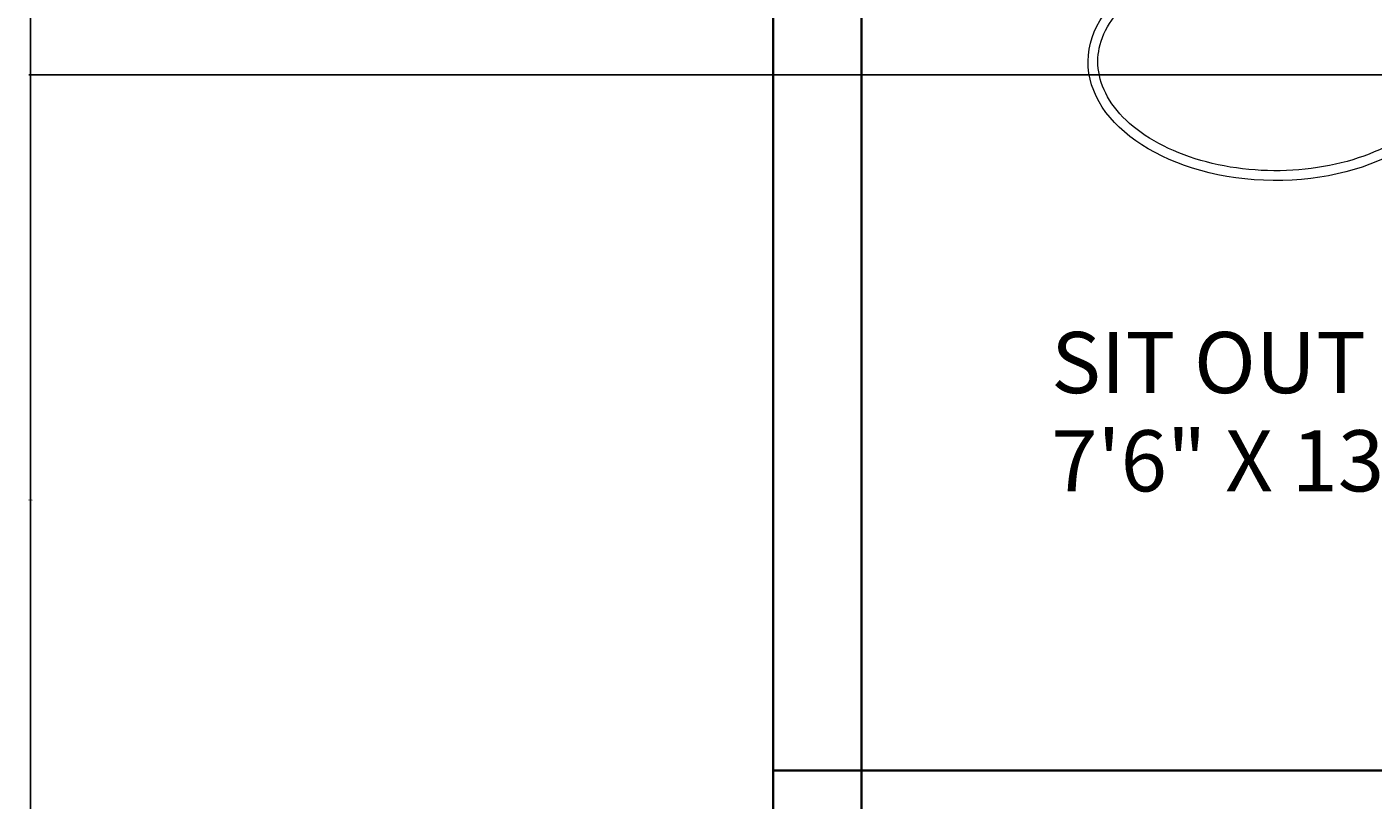
# Model space of a CAD drawing. Units: inches. Extents: x -61 to 1599, y -1316 to 257.
# Tile 14 of 204: x -61 to 76, y -947 to -868. Entities that reach past the tile are written whole.
import ezdxf

# ---------------------------------------------------------------- set-up
doc = ezdxf.new("R2010")
doc.units = ezdxf.units.IN
doc.header["$MEASUREMENT"] = 0
for name, color, linetype, lineweight in [('A-ANNO-DIMS', 2, 'Continuous', 18), ('A-AREA-IDEN', 1, 'Continuous', 18), ('FURNITURE', 83, 'Continuous', 18), ('WALLS', 4, 'Continuous', 35)]:
    doc.layers.add(name, color=color, linetype=linetype, lineweight=lineweight)
doc.styles.get("Standard").update_dxf_attribs({"font": 'arial.ttf'})
doc.dimstyles.get("Standard").update_dxf_attribs({"dimtxt": 0.18, "dimasz": 0.18, "dimexe": 0.18, "dimexo": 0.0625, "dimgap": 0.09, "dimtad": 0, "dimtih": 1, "dimtoh": 1, "dimdec": 0, "dimzin": 0, "dimdsep": 46, "dimlunit": 3, "dimtxsty": 'Standard', "dimcen": 0.09, "dimadec": 0, "dimazin": 0, "dimtfac": 1, "dimtdec": 0, "dimtofl": 0, "dimtmove": 0, "dimatfit": 3, "dimfxl": 1, "dimtolj": 1, "dimtzin": 0, "dimarcsym": 0})

# ---------------------------------------------------------------- blocks, each defined once
blk = doc.blocks.new('SIDE-TABLE-OVAL')
blk.add_ellipse((18.95, 11.99), major_axis=(-18.95, 0.16), ratio=0.632617)
blk.add_open_spline([(1, 12.14), (0.99, 11.17), (1.2, 10.2), (2.05, 8.28), (2.69, 7.34), (4.41, 5.58), (5.48, 4.76), (7.96, 3.32), (9.37, 2.71), (12.41, 1.74), (14.05, 1.4), (17.41, 1), (19.13, 0.95), (22.53, 1.15), (24.2, 1.41), (27.36, 2.19), (28.84, 2.73), (31.49, 4.02), (32.66, 4.78), (34.59, 6.45), (35.35, 7.36), (36.44, 9.24), (36.76, 10.2), (36.97, 12.14), (36.87, 13.11), (36.22, 15.04), (35.67, 16), (34.15, 17.81), (33.17, 18.67), (30.85, 20.19), (29.51, 20.86), (26.58, 21.94), (24.98, 22.36), (21.67, 22.89), (19.95, 23.01), (16.54, 22.94), (14.84, 22.76), (11.61, 22.1), (10.07, 21.63), (7.28, 20.44), (6.03, 19.73), (3.92, 18.13), (3.06, 17.25), (1.78, 15.4), (1.35, 14.44), (1.05, 13.03), (1, 12.59), (1, 12.14)], degree=3, knots=[0, 0, 0, 0, 0.279765, 0.279765, 0.559529, 0.559529, 0.839294, 0.839294, 1.119059, 1.119059, 1.398823, 1.398823, 1.678588, 1.678588, 1.958353, 1.958353, 2.238118, 2.238118, 2.517882, 2.517882, 2.797647, 2.797647, 3.077412, 3.077412, 3.357176, 3.357176, 3.636941, 3.636941, 3.916706, 3.916706, 4.19647, 4.19647, 4.476235, 4.476235, 4.756, 4.756, 5.035764, 5.035764, 5.315529, 5.315529, 5.595294, 5.595294, 5.875058, 5.875058, 6.154823, 6.154823, 6.283185, 6.283185, 6.283185, 6.283185])
blk = doc.blocks.new('*D687')
at = {"layer": 'A-ANNO-DIMS', "color": 0, "lineweight": -2, "transparency": 16777216}
for p, q in [((289.42, 181.68), (-61.08, 181.68)), ((-60.9, 181.5), (-60.9, -528.95)), ((-60.9, -1239.76), (-60.9, -529.32)), ((319.64, -1239.94), (-61.08, -1239.94))]:
    blk.add_line(p, q, dxfattribs=at)
at = {"layer": 'A-ANNO-DIMS', "color": 0, "transparency": 16777216}
for points in [[(-60.93, 181.5), (-60.87, 181.5), (-60.9, 181.68)], [(-60.93, -1239.76), (-60.87, -1239.76), (-60.9, -1239.94)]]:
    blk.add_solid(points, dxfattribs=at)
at = {"layer": 'DEFPOINTS', "color": 0, "transparency": 16777216}
for p in [(289.48, 181.68), (-60.9, -1239.94), (319.7, -1239.94)]:
    blk.add_point(p, dxfattribs=at)
at = {"layer": 'A-ANNO-DIMS', "color": 0, "transparency": 16777216, "insert": (-60.9, -529.13), "char_height": 0.18, "attachment_point": 5}
blk.add_mtext('\\A1;1421.6', dxfattribs=at)
blk = doc.blocks.new('*D693')
at = {"layer": 'A-ANNO-DIMS', "color": 0, "lineweight": -2, "transparency": 16777216}
for p, q in [((14.64, -616.94), (-61.08, -616.94)), ((-60.9, -617.12), (-60.9, -916.26)), ((-60.9, -1215.76), (-60.9, -916.63)), ((14.64, -1215.94), (-61.08, -1215.94))]:
    blk.add_line(p, q, dxfattribs=at)
at = {"layer": 'A-ANNO-DIMS', "color": 0, "transparency": 16777216}
for points in [[(-60.93, -617.12), (-60.87, -617.12), (-60.9, -616.94)], [(-60.93, -1215.76), (-60.87, -1215.76), (-60.9, -1215.94)]]:
    blk.add_solid(points, dxfattribs=at)
at = {"layer": 'DEFPOINTS', "color": 0, "transparency": 16777216}
for p in [(-60.9, -616.94), (14.7, -616.94), (14.7, -1215.94)]:
    blk.add_point(p, dxfattribs=at)
at = {"layer": 'A-ANNO-DIMS', "color": 0, "transparency": 16777216, "insert": (-60.9, -916.44), "char_height": 0.18, "attachment_point": 5}
blk.add_mtext('\\A1;599', dxfattribs=at)
blk = doc.blocks.new('*D696')
at = {"layer": 'A-ANNO-DIMS', "color": 0, "lineweight": -2, "transparency": 16777216}
for p, q in [((690.64, -873.17), (-61.08, -873.17)), ((-60.9, -873.35), (-60.9, -1025.8)), ((-60.9, -1178.61), (-60.9, -1026.16)), ((690.64, -1178.79), (-61.08, -1178.79))]:
    blk.add_line(p, q, dxfattribs=at)
at = {"layer": 'A-ANNO-DIMS', "color": 0, "transparency": 16777216}
for points in [[(-60.93, -873.35), (-60.87, -873.35), (-60.9, -873.17)], [(-60.93, -1178.61), (-60.87, -1178.61), (-60.9, -1178.79)]]:
    blk.add_solid(points, dxfattribs=at)
at = {"layer": 'DEFPOINTS', "color": 0, "transparency": 16777216}
for p in [(-60.9, -873.17), (690.7, -873.17), (690.7, -1178.79)]:
    blk.add_point(p, dxfattribs=at)
at = {"layer": 'A-ANNO-DIMS', "color": 0, "transparency": 16777216, "insert": (-60.9, -1025.98), "char_height": 0.18, "attachment_point": 5}
blk.add_mtext('\\A1;305.6', dxfattribs=at)

msp = doc.modelspace()

# ---------------------------------------------------------------- linework, layer by layer
at = {"layer": 'WALLS'}
for p, q in [((14.7028, -616.9446), (14.7028, -1215.9446)), ((23.7028, -943.9446), (23.7028, -787.9446)), ((14.7028, -943.9446), (234.7028, -943.9446)), ((23.7028, -943.9446), (23.7028, -1215.9446))]:
    msp.add_line(p, q, dxfattribs=at)

# ---------------------------------------------------------------- block references
at = {"layer": 'FURNITURE'}
msp.add_blockref('SIDE-TABLE-OVAL', (46.761, -883.9187), dxfattribs=at)

# ---------------------------------------------------------------- texts
at = {"layer": 'A-AREA-IDEN'}
for s, height, p in [('SIT OUT', 6.22364, (43.0043, -905.5446)), ('7\'6" X 13\'0"', 6.223643, (43.0043, -915.5424))]:
    msp.add_text(s, height=height, dxfattribs=at).set_placement(p)

# ---------------------------------------------------------------- dimensions: what is measured, and where the dimension line sits
at = {"layer": 'A-ANNO-DIMS'}
for base, p1, p2, override, picture, middle in [((-60.8972, -1239.9446), (289.4807, 181.6771), (319.7028, -1239.9446), {"dimdec": 1, "dimlfac": 1, "dimrnd": 0, "dimzin": 0, "dimdsep": 46, "dimlunit": 2}, '*D687', (-60.8972, -529.1337)), ((-60.8972, -616.9446), (14.7028, -1215.9446), (14.7028, -616.9446), {"dimdec": 0, "dimlfac": 1, "dimrnd": 0, "dimzin": 0, "dimdsep": 46, "dimlunit": 2}, '*D693', (-60.8972, -916.4446)), ((-60.8972, -873.169), (690.7028, -1178.7933), (690.7028, -873.169), {"dimdec": 1, "dimlfac": 1, "dimrnd": 0, "dimzin": 0, "dimdsep": 46, "dimlunit": 2}, '*D696', (-60.8972, -1025.9812))]:
    dim = msp.add_linear_dim(base=base, p1=p1, p2=p2, angle=90, dimstyle='Standard', override=override, dxfattribs=at)
    dim.commit()
    dim.dimension.update_dxf_attribs({"geometry": picture, "text_midpoint": middle})

doc.saveas('drawing.dxf')
